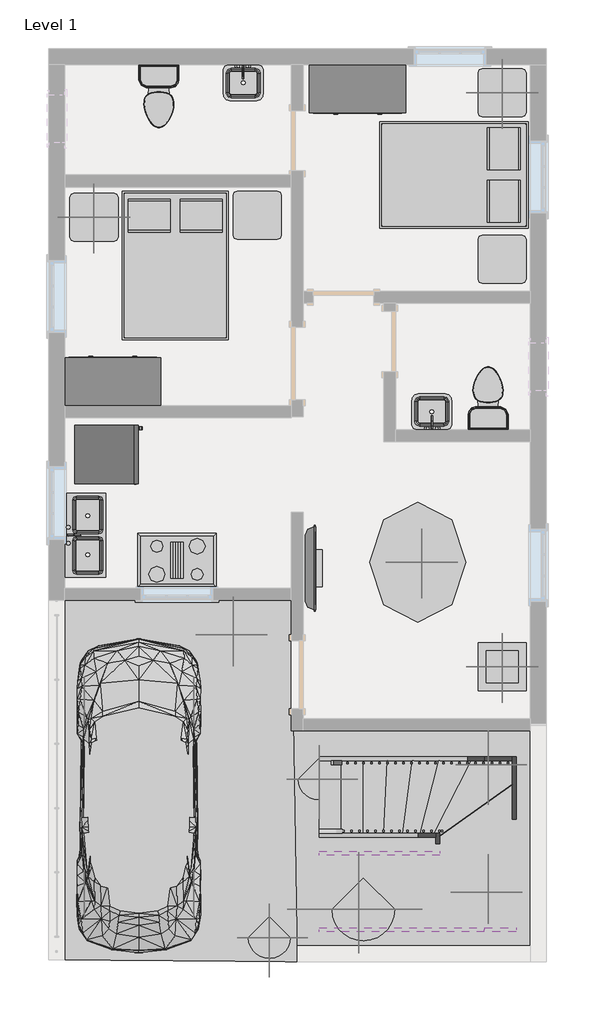
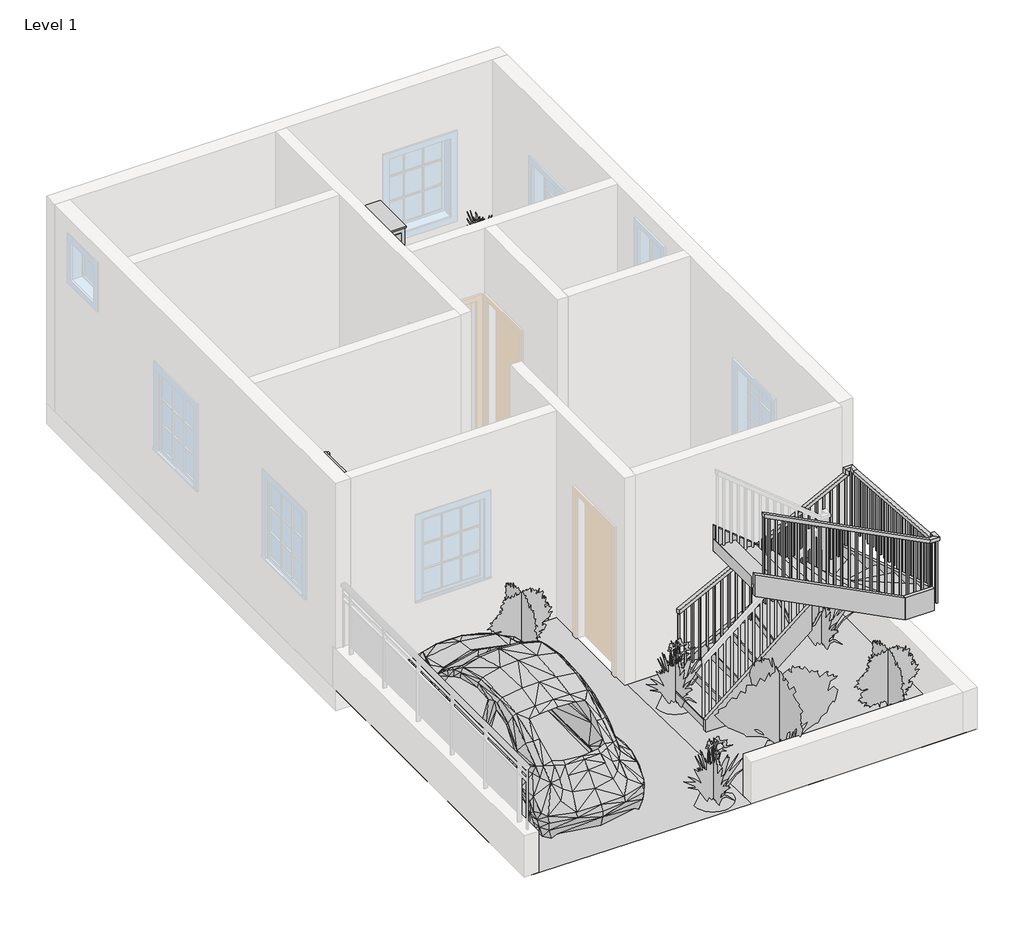
# One storey, part 2 of 2: 11 furniture elements, 10 geographic elements, 8 members, 7 flow terminals, 5 proxies, 1 railing, 1 stair flight.
# Revit data of these elements (continued)
# Element 10 (IfcFlowTerminal, "Sink Vanity-Square : 20\" x 18\"")
#   Mark = "5"
#   Phase Created = New Construction
#   Materials on its faces: "Porcelain, Linen", "Steel, Polished"
# Element 11 (IfcFlowTerminal, "Toilet-Domestic-3D : Toilet-Domestic-3D")
#   Mark = "1"
#   Phase Created = New Construction
#   Materials on its faces: "Porcelain, Linen", "Laminate, Linen, Matte"
# Element 12 (IfcFlowTerminal, "Toilet-Domestic-3D : Toilet-Domestic-3D")
#   Mark = "4"
#   Phase Created = New Construction
#   Materials on its faces: "Porcelain, Linen", "Laminate, Linen, Matte"
# Elements 13, 14 (IfcFurniture, "Bed-Box : Double 53\" x 74\"")
#   Phase Created = New Construction
#   Materials on its faces: "Birch", "Linen, White"
# Elements 15, 16 (IfcFurniture, "Dresser : 48\" x 60\" x 24\"")
#   Phase Created = New Construction
#   Materials on its faces: "Laminate, Ivory, Matte", "Cherry", "Laminate - Ivory, Glossy"
# Element 17 (IfcFurniture, "TV - Flat Screen : 42\"")
#   Stand = yes
#   Phase Created = New Construction
#   Materials on its faces: "TV - Black", "TV - Glass", "TV - Screen"
# Element 18 (IfcFurniture, "Table-Coffee : 24\" x 24\" x 24\"")
#   Phase Created = New Construction
#   Materials on its faces: "Glass - Clear, Grey"
# Element 19 (IfcFurniture, "Table-Ellipse : 60\" x 48\"")
#   Phase Created = New Construction
#   Materials on its faces: "Birch"
# Elements 20, 21, 22, 23 (IfcFurniture, "Table-End : 24\" x 24\"")
#   Phase Created = New Construction
#   Materials on its faces: "Laminate, Ivory, Matte", "Birch"
# Elements 24, 25, 26, 27 (IfcGeographicElement, "RPC Plant - Tropical")
#   Phase Created = New Construction
# Elements 28, 29, 30, 31 (IfcGeographicElement, "RPC Plant - Tropical : Agave - 1.5'")
#   Phase Created = New Construction
# Elements 32, 33 (IfcGeographicElement, "RPC Plant - Tropical : Jungle Flame - 3'")
#   Phase Created = New Construction
# Elements 34, 35, 36, 37, 38, 39, 40, 41 (IfcMember, "Stringer - 2\" Width")
#   Phase Created = New Construction
# Element 42 (IfcRailing, "Handrail - Rectangular")
#   Phase Created = New Construction
# Element 43 (IfcStairFlight, "2\" Tread 1\" Nosing 1/4\" Riser")
#   Phase Created = New Construction
# Materials
#   "Steel, Chrome Plated": class "Metal", colour RGB 17 17 17, transparency 0, Description = "Chromiuim plated steel", Cost = 0
#   "Steel, Polished": class "Metal", colour RGB 57 57 57, transparency 0, Description = "Polished steel", Cost = 0
#   "Steel, Paint Finish, Ivory, Glossy": class "Metal", colour RGB 247 247 239, transparency 0, Description = "Steel, paint finish, ivory, glossy", Cost = 0
#   "Porcelain, Linen": class "Ceramic", colour RGB 249 239 230, transparency 0, Description = "Porcelain, linen", Cost = 0
#   "Laminate, Linen, Matte": class "Plastic", colour RGB 249 239 230, transparency 0, Description = "Plastic Laminate - Linen, Matte", Cost = 0
#   "Birch": class "Wood", colour RGB 224 178 126, transparency 0, Description = "Betula Alleghaniensis", Cost = 0
#   "Linen, White": class "Textile", colour RGB 247 247 239, transparency 0, Description = "Linen, white", Cost = 0
#   "Laminate - Ivory, Glossy": colour RGB 247 247 239, transparency 0
#   "Laminate, Ivory, Matte": class "Plastic", colour RGB 247 247 239, transparency 0, Description = "Plastic Laminate - Ivory, Matte", Cost = 0
#   "Cherry": class "Wood", colour RGB 226 177 128, transparency 0, Description = "Prunus Serotina", Cost = 0
#   "TV - Black": colour RGB 49 49 49, transparency 0
#   "TV - Glass": colour RGB 157 157 157, transparency 0.9
#   "TV - Screen": colour RGB 0 0 0, transparency 0
#   "Glass - Clear, Grey": class "Glass", colour RGB 252 255 255, transparency 0.64
